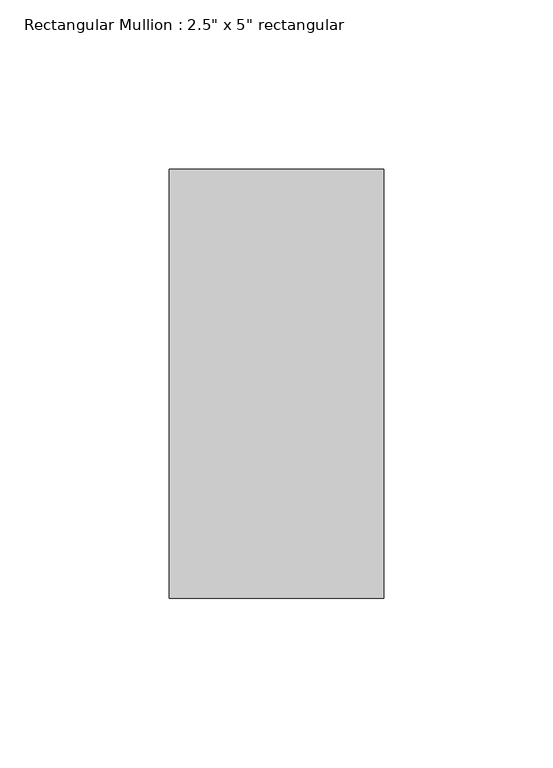
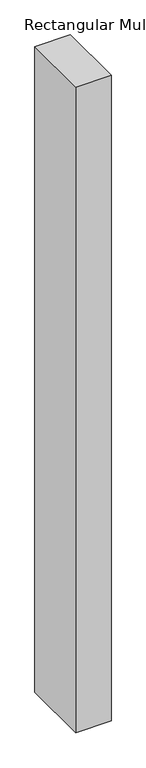
"""IFC4 building model written with IfcOpenShell, lengths in millimetres: member geometry."""

from ifc_helpers import new_model, si_unit, frame, origin, place, context, project, spatial, polyline, outline, extrude, source, transform, mapped, element, save


def member_5a365947(model_context):
    return source(origin(), model_context, "Body", "SweptSolid", [
        extrude(outline(polyline([(0.0, 63.5), (0.0, -63.5), (-63.5, -63.5), (-63.5, 63.5), (0.0, 63.5)])), frame((0.0, 0.0, -1227.57546), z_axis=(0.0, 0.0, 1.0), x_axis=(1.0, 0.0, 0.0)), (0.0, 0.0, 1.0), 1227.57546),
    ])


if __name__ == "__main__":
    model = new_model("IFC4")
    model_context = context("Model", 3, world=origin())
    ifc_project = project(units=[si_unit("LENGTHUNIT", "METRE", prefix="MILLI")], contexts=[model_context])
    site = spatial("IfcSite", under=ifc_project)
    building = spatial("IfcBuilding", under=site)
    placement = place(None, origin())
    member_shape = member_5a365947(model_context)
    element("IfcMember", 1, ObjectType="Rectangular Mullion : 2.5\" x 5\" rectangular", at=placement, inside=building, context=model_context, shape_type="MappedRepresentation", body=[
        mapped(member_shape, transform((0.0, 0.0, 0.0), x_axis=(1.0, 0.0, 0.0), y_axis=(0.0, 1.0, 0.0), z_axis=(0.0, 0.0, 1.0))),
    ])
    save(model, "model.ifc")

# Revit data of these elements
# Type "Rectangular Mullion : 2.5\" x 5\" rectangular"
#   built-in parameter 1007304 = 0.416667 (stored number, unit not read)
#   built-in parameter 1007301 = 0.104167 (stored number, unit not read)
#   built-in parameter 1007300 = 0.104167 (stored number, unit not read)
# Element 1 (IfcMember, "Rectangular Mullion : 2.5\" x 5\" rectangular")
#   Materials on its faces: "Iron, Ductile"
# Materials
#   "Iron, Ductile": class "Metal", colour RGB 0 0 0, transparency 0, Description = "Ductile cast iron", Cost = 0
